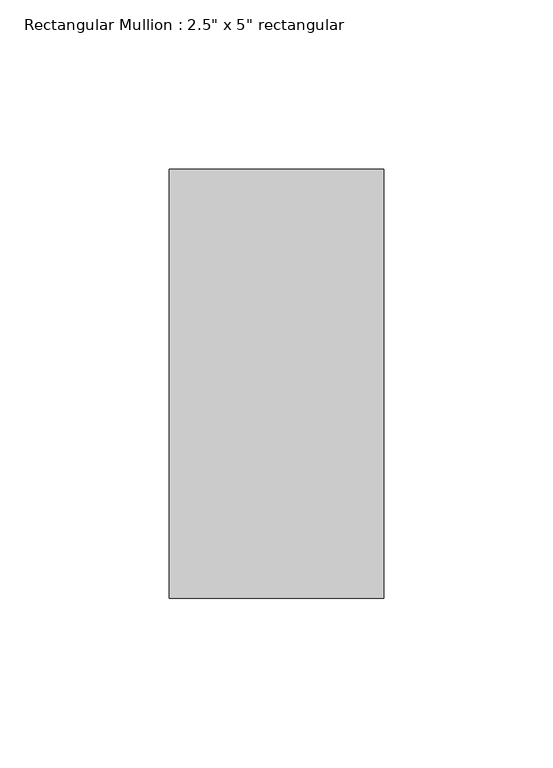
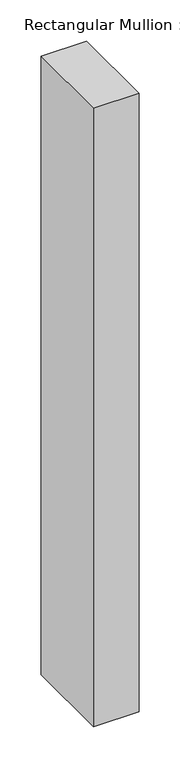
"""IFC4 building model written with IfcOpenShell, lengths in millimetres: member geometry."""

from ifc_helpers import new_model, si_unit, frame, origin, place, context, project, spatial, polyline, outline, extrude, source, transform, mapped, element, save


def member_c9167585(model_context):
    return source(origin(), model_context, "Body", "SweptSolid", [
        extrude(outline(polyline([(0.0, 63.5), (0.0, -63.5), (-63.5, -63.5), (-63.5, 63.5), (0.0, 63.5)])), frame((0.0, 0.0, -913.799557), z_axis=(0.0, 0.0, 1.0), x_axis=(1.0, 0.0, 0.0)), (0.0, 0.0, 1.0), 913.799557),
    ])


if __name__ == "__main__":
    model = new_model("IFC4")
    model_context = context("Model", 3, world=origin())
    ifc_project = project(units=[si_unit("LENGTHUNIT", "METRE", prefix="MILLI")], contexts=[model_context])
    site = spatial("IfcSite", under=ifc_project)
    building = spatial("IfcBuilding", under=site)
    placement = place(None, origin())
    member_shape = member_c9167585(model_context)
    element("IfcMember", 1, ObjectType="Rectangular Mullion : 2.5\" x 5\" rectangular", at=placement, inside=building, context=model_context, shape_type="MappedRepresentation", body=[
        mapped(member_shape, transform((0.0, 0.0, 0.0), x_axis=(1.0, 0.0, 0.0), y_axis=(0.0, 1.0, 0.0), z_axis=(0.0, 0.0, 1.0))),
    ])
    save(model, "model.ifc")

# Revit data of these elements
# Type "Rectangular Mullion : 2.5\" x 5\" rectangular"
#   built-in parameter 1007304 = 0.416667 (stored number, unit not read)
#   built-in parameter 1007301 = 0.104167 (stored number, unit not read)
#   built-in parameter 1007300 = 0.104167 (stored number, unit not read)
# Element 1 (IfcMember, "Rectangular Mullion : 2.5\" x 5\" rectangular")
#   Materials on its faces: "Aluminum"
# Materials
#   "Aluminum": class "Metal", colour RGB 247 247 247, transparency 0, Description = "Aluminum 6061", Cost = 0
